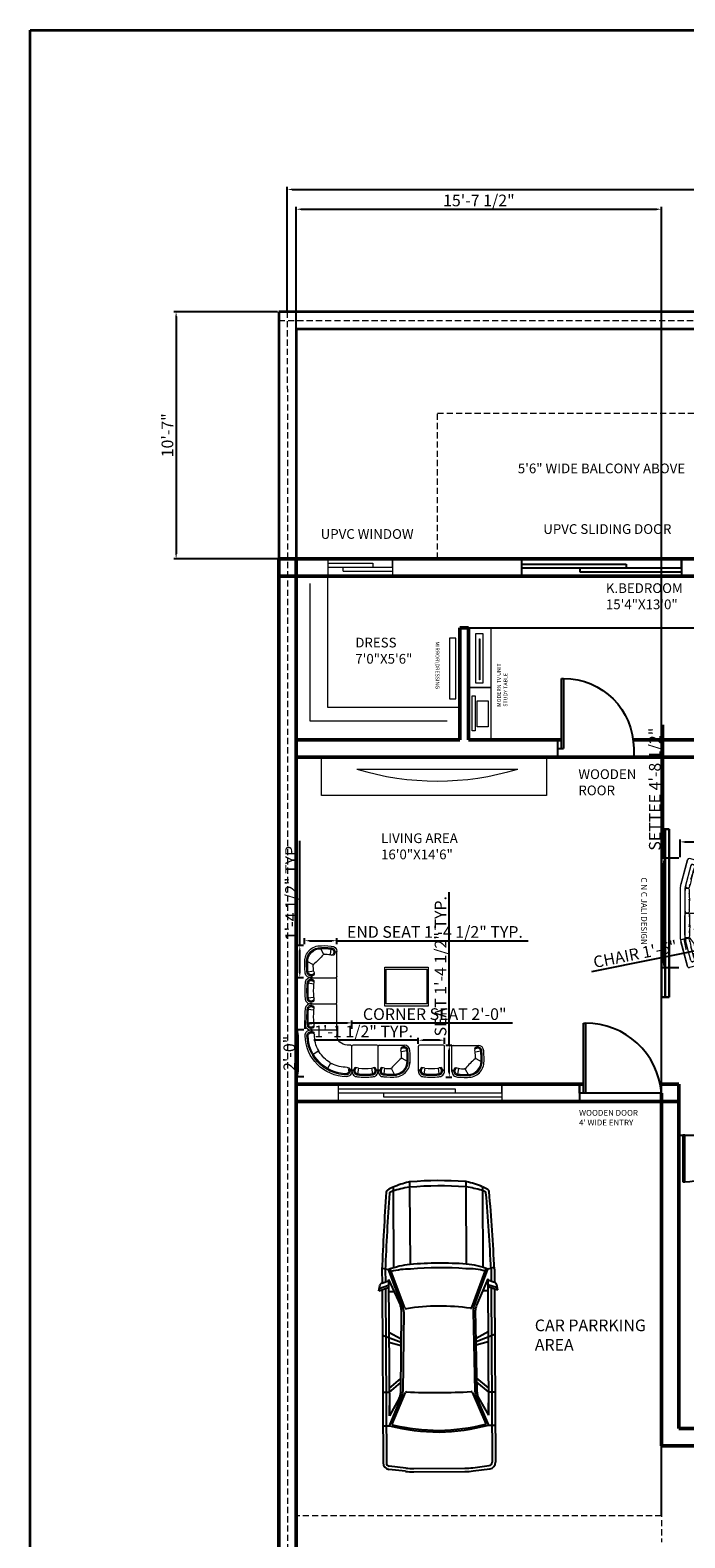
# Model space of a CAD drawing. Units: inches. Extents: x 2123 to 2977, y 1464 to 2698.
# Tile 2 of 10: x 2123 to 2459, y 1923 to 2698. Entities that reach past the tile are written whole.
import ezdxf

# ---------------------------------------------------------------- set-up
doc = ezdxf.new("R2010")
doc.units = ezdxf.units.IN
doc.linetypes.add('HIDDEN2', pattern=[4.7625, 3.175, -1.5875])
doc.layers.add('0 finos', color=250, linetype='Continuous')
for name, color, linetype, lineweight in [('A-ANNO-DIMS', 2, 'Continuous', 18), ('A-ANNO-TEXT', 7, 'Continuous', 18), ('A-ANNO-TTLB', 7, 'Continuous', 35), ('A-AREA-IDEN', 7, 'Continuous', 25), ('A-DOOR', 4, 'Continuous', 25), ('A-FLOR-OVHD', 253, 'HIDDEN2', 18), ('A-FURN', 8, 'Continuous', 18), ('A-FURN-FIXD', 8, 'Continuous', 20), ('A-GLAZ', 4, 'Continuous', 18), ('A-WALL', 7, 'Continuous', 50), ('A-WALL-PRTN', 7, 'Continuous', 30), ('C-PKNG-VEHC', 8, 'Continuous', 18), ('C-PROP', 21, 'HIDDEN2', 18), ('L-SITE-WALL', 7, 'Continuous', 35)]:
    doc.layers.add(name, color=color, linetype=linetype, lineweight=lineweight)
doc.styles.get("Standard").update_dxf_attribs({"font": 'arial.ttf'})
doc.dimstyles.new('ISO-25', dxfattribs={"dimtxt": 6, "dimasz": 2.5, "dimexe": 1.25, "dimexo": 0.625, "dimtad": 1, "dimdec": 0, "dimlunit": 3, "dimtxsty": 'Standard', "dimcen": 2.5, "dimadec": 0, "dimazin": 0, "dimtfac": 1, "dimtdec": 0, "dimtmove": 0, "dimatfit": 3, "dimfxl": 1, "dimarcsym": 0})

# ---------------------------------------------------------------- blocks, each defined once
blk = doc.blocks.new('carro')
at = {"layer": '0 finos'}
for p, q in [((-1.274, 0.841), (-1.249, 0.743)), ((-0.666, 0.502), (-1.258, 0.718)), ((-0.674, 0.532), (-1.249, 0.743)), ((-1.246, 0.843), (-1.047, 0.844)), ((-1.246, 0.793), (-1.063, 0.794)), ((-1.099, 0.744), (0.965, 0.756)), ((-1.099, 0.744), (-0.702, 0.571)), ((-1.045, 0.847), (-1.079, 0.744)), ((-0.964, 0.889), (-1.011, 0.744)), ((-0.93, 0.895), (-1.007, 0.881)), ((-0.93, 0.895), (-0.979, 0.744)), ((-0.963, 0.794), (1.676, 0.81)), ((-0.947, 0.845), (1.676, 0.86)), ((-0.919, 0.745), (-0.919, 0.665)), ((-0.299, 0.748), (-0.198, 0.565)), ((-0.258, 0.849), (-0.148, 0.566)), ((-0.149, 0.749), (-0.098, 0.567)), ((0.551, 0.753), (0.402, 0.577)), ((0.61, 0.754), (0.462, 0.578)), ((0.61, 0.754), (0.609, 0.854)), ((0.616, 0.508), (1.094, 0.714)), ((0.669, 0.564), (1.115, 0.756)), ((0.701, 0.605), (0.965, 0.756)), ((0.965, 0.756), (0.778, 0.755)), ((1.115, 0.756), (1.114, 0.856)), ((1.759, 0.516), (1.726, 0.766)), ((1.809, 0.522), (1.776, 0.773)), ((-2.494, 0.661), (-2.439, 0.661)), ((-2.439, 0.661), (-1.275, 0.668)), ((0.615, 0.581), (-0.626, 0.557)), ((-0.608, 0.521), (0.602, 0.549)), ((-2.573, 0.41), (-2.493, 0.411)), ((-2.476, 0.411), (-1.323, 0.417)), ((1.771, -0.377), (1.767, 0.398)), ((1.821, -0.377), (1.817, 0.398)), ((-2.568, -0.44), (-2.488, -0.439)), ((-2.471, -0.439), (-1.318, -0.433)), ((-2.432, -0.689), (-1.267, -0.682)), ((-0.661, -0.51), (-1.25, -0.733)), ((-0.668, -0.54), (-1.241, -0.757)), ((-1.091, -0.756), (-0.695, -0.579)), ((-0.911, -0.755), (-0.911, -0.676)), ((0.622, -0.574), (-0.62, -0.564)), ((-0.602, -0.528), (0.608, -0.542)), ((-0.291, -0.752), (-0.192, -0.567)), ((-0.248, -0.851), (-0.142, -0.568)), ((-0.141, -0.751), (-0.092, -0.568)), ((0.559, -0.747), (0.408, -0.572)), ((0.619, -0.746), (0.468, -0.573)), ((1.102, -0.701), (0.622, -0.501)), ((1.124, -0.743), (0.676, -0.556)), ((0.708, -0.597), (0.974, -0.744)), ((1.765, -0.495), (1.735, -0.746)), ((1.814, -0.501), (1.785, -0.752)), ((-2.487, -0.689), (-2.432, -0.689)), ((-1.262, -0.856), (-1.241, -0.757)), ((-1.237, -0.807), (-1.054, -0.806)), ((-1.236, -0.857), (-1.037, -0.856)), ((-1.091, -0.756), (0.974, -0.744)), ((-1.036, -0.859), (-1.071, -0.756)), ((-0.953, -0.9), (-1.002, -0.756)), ((-0.92, -0.905), (-0.996, -0.892)), ((-0.92, -0.905), (-0.971, -0.756)), ((-0.954, -0.806), (1.686, -0.79)), ((-0.937, -0.855), (1.686, -0.84)), ((0.619, -0.746), (0.619, -0.846)), ((0.974, -0.744), (0.819, -0.745)), ((1.124, -0.843), (1.124, -0.743))]:
    blk.add_line(p, q, dxfattribs=at)
for centre, radius, start, end in [((-2.14, 0.534), 0.376, 145.8602, 160.2963), ((-2.414, 0.72), 0.045, 99.6056, 145.8602), ((-2.25, 0.596), 0.2, 150.5092, 164.4728), ((-2.14, 0.534), 0.326, 147.5998, 150.5092), ((0.535, -34.533), 35.421, 92.8817, 94.7876), ((-2.403, 0.7), 0.015, 94.7595, 147.5998), ((0.535, -34.583), 35.421, 92.8817, 94.7595), ((-0.078, 0.306), 1.25, 159.5351, 174.8753), ((-0.049, 0.42), 1.205, 166.3495, 180.3763), ((-0.998, 0.832), 0.05, 100.189, 161.8979), ((1.096, 0.709), 0.005, 13.9297, 113.3542), ((-2.008, -0.06), 3.203, 1.1964, 13.9297), ((-2.008, -0.06), 3.228, 1.1964, 14.6587), ((1.677, 0.76), 0.1, 7.4579, 90.3329), ((1.677, 0.76), 0.05, 7.4579, 90.3329), ((-1.339, 0.159), 1.259, 156.5474, 167.8615), ((-0.601, 0.138), 1.911, 164.4728, 171.5741), ((-0.63, 0.737), 0.18, 246.5804, 271.1487), ((2.517, 0.015), 3.205, 171.6477, 189.0181), ((-0.612, 0.701), 0.18, 249.9002, 271.3224), ((-0.673, 0.483), 0.02, 351.6477, 69.9002), ((0.598, 0.729), 0.18, 271.3224, 293.3542), ((0.622, 0.494), 0.015, 113.3542, 183.6852), ((-5.6, 0.093), 6.22, 359.1748, 3.6852), ((0.612, 0.761), 0.18, 271.1487, 299.704), ((0.817, 0.392), 0.95, 0.3329, 7.4579), ((0.817, 0.392), 1, 0.3329, 7.4579), ((2.688, 0.016), 5.275, 175.8587, 184.807), ((-2.375, 0.382), 0.2, 167.8615, 175.8587), ((2.688, 0.016), 5.195, 175.7191, 184.9467), ((-2.294, 0.389), 0.2, 171.5741, 175.7191), ((3.848, 0.022), 5.186, 175.6321, 185.0337), ((3.848, 0.022), 5.116, 175.6321, 185.0337), ((-5.599, -0.158), 6.22, 356.9806, 1.4909), ((-2.008, 0.037), 3.203, 346.7361, 359.4694), ((-2.008, 0.037), 3.228, 346.0071, 359.4694), ((-2.37, -0.41), 0.2, 184.807, 192.8043), ((-1.337, -0.175), 1.259, 192.8043, 204.1184), ((-2.289, -0.415), 0.2, 184.9467, 189.0917), ((-0.6, -0.145), 1.911, 189.0917, 196.7185), ((-0.074, -0.307), 1.25, 185.7904, 201.1307), ((-0.044, -0.42), 1.205, 180.2895, 194.3163), ((0.822, -0.383), 0.95, 353.2079, 0.3329), ((0.822, -0.383), 1, 353.2079, 0.3329), ((-0.621, -0.744), 0.18, 89.5171, 114.0853), ((-0.604, -0.708), 0.18, 89.3433, 110.7656), ((-0.668, -0.491), 0.02, 290.7656, 9.0181), ((0.606, -0.722), 0.18, 67.3115, 89.3433), ((0.628, -0.487), 0.015, 176.9806, 247.3115), ((0.621, -0.754), 0.18, 60.9617, 89.5171), ((-2.134, -0.558), 0.376, 200.3694, 214.8056), ((-2.406, -0.748), 0.045, 214.8056, 261.0602), ((-2.406, -0.687), 0.025, 196.7185, 205.3192), ((-2.134, -0.558), 0.326, 205.3192, 213.066), ((0.133, 34.537), 35.421, 265.8782, 267.7841), ((-2.395, -0.728), 0.015, 213.066, 265.9063), ((0.133, 34.587), 35.421, 265.9063, 267.7841), ((-0.988, -0.843), 0.05, 198.7678, 260.4768), ((1.104, -0.697), 0.005, 247.3115, 346.7361), ((1.685, -0.74), 0.05, 270.3329, 353.2079), ((1.685, -0.74), 0.1, 270.3329, 353.2079)]:
    blk.add_arc(centre, radius, start, end, dxfattribs=at)
blk = doc.blocks.new('ДИВАН08')
for p, q in [((10, 838), (233, 1669)), ((233, 1669), (26, 897)), ((339, 1486), (160, 818)), ((777, 1575), (294, 1705)), ((1026, 1343), (400, 1521)), ((691, 1435), (619, 1433)), ((812, 1514), (787, 1417)), ((400, 1260), (453, 1348)), ((540, 1030), (740, 1020)), ((550, 1060), (830, 950)), ((910, 720), (1061, 1282)), ((0, 761), (0, -761)), ((150, 741), (150, -741)), ((480, 400), (800, 500)), ((900, 642), (900, -642)), ((310, 0), (900, 0)), ((780, 460), (580, 470)), ((600, -460), (430, -520)), ((10, -838), (233, -1669)), ((233, -1669), (26, -897)), ((339, -1486), (160, -818)), ((430, -500), (800, -530)), ((910, -720), (1061, -1282)), ((400, -1260), (453, -1348)), ((1026, -1343), (400, -1521)), ((500, -1100), (840, -1040)), ((800, -1020), (620, -1120)), ((777, -1575), (294, -1705)), ((691, -1435), (619, -1433)), ((812, -1514), (787, -1417))]:
    blk.add_line(p, q)
for centre, radius, start, end in [((281, 1656), 50, 75, 165), ((387, 1473), 50, 75, 165), ((362, 1495), 20, 89.0297, 94.7193), ((359, 1330), 185, 60.9703, 89.0297), ((439, 1474), 20, 345, 60.9703), ((764, 1527), 50, 345, 75), ((-610, 1509), 1045, 334.4223, 341.4421), ((298, 1228), 90.2, 326.9449, 350.757), ((1013, 1295), 50, 345, 75), ((300, 761), 300, 165, 180), ((450, 741), 300, 165, 180), ((242, 847), 72.2, 156.1517, 210.7358), ((269, 972), 185, 240.9703, 269.0297), ((266, 807), 20, 269.0297, 345), ((-57, 544), 353, 1.9165, 10.4824), ((213, 880), 92.8, 338.027, 9.0149), ((1200, 642), 300, 165, 180), ((86, 55), 209, 1.7155, 15.9571), ((-23, 353), 322, 358.4137, 13.7556), ((86, -55), 209, 344.0429, 358.2845), ((-23, -353), 322, 346.2444, 1.5863), ((300, -761), 300, 180, 195), ((450, -741), 300, 180, 195), ((242, -847), 72.2, 149.2642, 203.8483), ((269, -972), 185, 90.9703, 119.0297), ((266, -807), 20, 15, 90.9703), ((-57, -544), 353, 349.5176, 358.0835), ((213, -880), 92.8, 350.9851, 21.973), ((1200, -642), 300, 180, 195), ((-610, -1509), 1045, 18.5579, 25.5777), ((298, -1228), 90.2, 9.243, 33.0551), ((1013, -1295), 50, 285, 15), ((281, -1656), 50, 195, 285), ((387, -1473), 50, 195, 285), ((362, -1495), 20, 265.2807, 270.9703), ((359, -1330), 185, 270.9703, 299.0297), ((439, -1474), 20, 299.0297, 15), ((764, -1527), 50, 285, 15)]:
    blk.add_arc(centre, radius, start, end)
for points, knots in [([(459, 1469), (452, 1440), (431, 1359), (378, 1199), (347, 1000), (304, 860), (286, 801)], [0, 0, 0, 0, 90.187713, 250.973361, 505.38742, 689.989893, 689.989893, 689.989893, 689.989893]), ([(398, 1251), (413, 1308), (433, 1384), (489, 1480), (588, 1481), (651, 1453), (691, 1435)], [0, 0, 0, 0, 182.307841, 236.159489, 312.31722, 446.240501, 446.240501, 446.240501, 446.240501]), ([(525, 1401), (539, 1407), (583, 1425), (652, 1391), (683, 1425), (691, 1435)], [0, 0, 0, 0, 44.660676, 140.870988, 176.926501, 176.926501, 176.926501, 176.926501]), ([(400, 1260), (417, 1265), (477, 1281), (481, 1367), (520, 1397), (525, 1401)], [0, 0, 0, 0, 50, 176.134878, 196.761653, 196.761653, 196.761653, 196.761653]), ([(156, 55), (155, 68), (151, 132), (151, 244), (150, 392), (154, 520), (148, 633), (153, 704), (162, 778), (223, 769), (278, 775), (303, 714), (290, 642), (303, 516), (300, 345), (298, 186), (295, 82), (296, 27), (255, 6), (217, 1), (173, 12), (157, 41), (156, 55)], [0, 0, 0, 0, 37.52683, 194.502639, 336.34661, 480.520736, 579.37384, 668.990026, 713.725273, 764.098689, 821.099919, 865.09763, 933.523372, 1043.042771, 1240.322997, 1451.300934, 1509.736774, 1565.888367, 1594.82446, 1636.840587, 1680.06496, 1722.682399, 1722.682399, 1722.682399, 1722.682399]), ([(156, -55), (155, -68), (151, -132), (151, -244), (150, -392), (154, -520), (148, -633), (153, -704), (162, -778), (223, -769), (278, -775), (303, -714), (290, -642), (303, -516), (300, -345), (298, -186), (295, -82), (296, -27), (255, -6), (217, -1), (173, -12), (157, -41), (156, -55)], [0, 0, 0, 0, 37.52683, 194.502639, 336.34661, 480.520736, 579.37384, 668.990026, 713.725273, 764.098689, 821.099919, 865.09763, 933.523372, 1043.042771, 1240.322997, 1451.300934, 1509.736774, 1565.888367, 1594.82446, 1636.840587, 1680.06496, 1722.682399, 1722.682399, 1722.682399, 1722.682399]), ([(459, -1469), (452, -1440), (431, -1359), (378, -1199), (347, -1000), (304, -860), (286, -801)], [0, 0, 0, 0, 90.187713, 250.973361, 505.38742, 689.989893, 689.989893, 689.989893, 689.989893]), ([(398, -1251), (413, -1308), (433, -1384), (489, -1480), (588, -1481), (651, -1453), (691, -1435)], [0, 0, 0, 0, 182.307841, 236.159489, 312.31722, 446.240501, 446.240501, 446.240501, 446.240501]), ([(400, -1260), (417, -1265), (477, -1281), (481, -1367), (520, -1397), (525, -1401)], [0, 0, 0, 0, 50, 176.134878, 196.761653, 196.761653, 196.761653, 196.761653]), ([(525, -1401), (539, -1407), (583, -1425), (652, -1391), (683, -1425), (691, -1435)], [0, 0, 0, 0, 44.660676, 140.870988, 176.926501, 176.926501, 176.926501, 176.926501])]:
    blk.add_open_spline(points, degree=3, knots=knots)
blk = doc.blocks.new('A$C707258B2')
at = {"color": 0}
for p, q in [((0.404, 0.342), (1.074, 0.342)), ((0.404, 0.292), (0.454, 0.292)), ((0.404, 0.262), (0.454, 0.262)), ((1.104, 0.312), (1.104, 0.212)), ((0.6, -0.238), (0.47, -0.313)), ((1.479, -0.063), (1.379, -0.063)), ((1.509, -0.763), (1.509, -0.093)), ((0.929, -0.567), (0.854, -0.697)), ((1.429, -0.763), (1.429, -0.713)), ((1.459, -0.763), (1.459, -0.712))]:
    blk.add_line(p, q, dxfattribs=at)
for centre, radius, start, end in [((0.404, 0.192), 0.15, 90, 181.1754), ((1.379, 0.212), 1.125, 181.1754, 268.8246), ((0.404, 0.192), 0.1, 90, 181.1754), ((1.379, 0.212), 1.075, 181.1754, 208.6357), ((0.404, 0.192), 0.07, 90, 181.1754), ((1.379, 0.212), 1.045, 181.1754, 268.8246), ((0.378, 0.317), 0.0362, 316.3972, 43.6028), ((0.368, 0.317), 0.0662, 337.8298, 22.1702), ((0.455, 0.256), 0.0357, 345.4262, 90.5555), ((0.454, 0.212), 0.05, 360, 90), ((1.379, 0.212), 0.875, 180, 208.4082), ((1.074, 0.312), 0.03, 360, 90), ((1.379, 0.212), 0.275, 180, 270), ((0.457, -0.291), 0.025, 208.6357, 300), ((0.482, -0.334), 0.025, 120, 211.3643), ((1.379, 0.212), 1.075, 211.3643, 238.6357), ((0.587, -0.216), 0.025, 300, 28.4082), ((0.612, -0.259), 0.025, 31.5918, 120), ((1.379, 0.212), 0.875, 211.5918, 238.4082), ((1.479, -0.093), 0.03, 360, 90), ((0.832, -0.685), 0.025, 238.6357, 330), ((0.876, -0.71), 0.025, 150, 241.3643), ((1.379, 0.212), 1.075, 241.3643, 268.8246), ((0.907, -0.555), 0.025, 330, 58.4082), ((0.951, -0.58), 0.025, 61.5918, 150), ((1.379, 0.212), 0.875, 241.5918, 270), ((1.359, -0.763), 0.15, 268.8246, 360), ((1.359, -0.763), 0.1, 268.8246, 360), ((1.359, -0.763), 0.07, 268.8246, 360), ((1.379, -0.713), 0.05, 360, 90), ((1.425, -0.709), 0.0336, 354.6301, 109.3883), ((1.484, -0.799), 0.0662, 67.8298, 112.1702), ((1.484, -0.789), 0.0362, 46.3972, 133.6028)]:
    blk.add_arc(centre, radius, start, end, dxfattribs=at)
blk = doc.blocks.new('part 01')
at = {"color": 0}
for p, q in [((-591, 527), (-740, 550)), ((-670, 700), (0, 700)), ((-591, 527), (-579, 561)), ((30, 30), (30, 670)), ((-591, 173), (-740, 150)), ((-670, 0), (0, 0)), ((-591, 173), (-579, 139))]:
    blk.add_line(p, q, dxfattribs=at)
for centre, radius, start, end in [((1178, 350), 2008, 174.2835, 185.7165), ((-670, 550), 150, 90, 181.1754), ((1178, 350), 1958, 174.2835, 185.7165), ((-670, 550), 100, 90, 181.1754), ((1178, 350), 1928, 174.2835, 185.7165), ((-670, 550), 70, 90, 181.1754), ((-660, 518), 133, 56.0897, 95.6132), ((-696, 675), 36.2, 316.3972, 43.6028), ((-660, 518), 103, 42.0066, 95.6132), ((-706, 675), 66.2, 337.8298, 22.1702), ((1178, 350), 1778, 174.2835, 185.7165), ((-600, 607), 25, 332.9608, 56.0897), ((-625, 620), 53.2, 321.0017, 332.9608), ((-602, 570), 25, 340, 42.0066), ((0, 670), 30, 0, 90), ((-670, 150), 150, 178.8246, 270), ((-670, 150), 100, 178.8246, 270), ((-670, 150), 70, 178.8246, 270), ((-660, 182), 133, 264.3868, 303.9103), ((-660, 182), 103, 264.3868, 317.9934), ((-696, 25), 36.2, 316.3972, 43.6028), ((-706, 25), 66.2, 337.8298, 22.1702), ((-600, 93), 25, 303.9103, 27.0392), ((-602, 130), 25, 317.9934, 20), ((-625, 80), 53.2, 27.0392, 38.9983), ((0, 30), 30, 270, 0)]:
    blk.add_arc(centre, radius, start, end, dxfattribs=at)
blk = doc.blocks.new('part02')
at = {"color": 0}
for p, q in [((0, -670), (0, 0)), ((30, 30), (700, 30)), ((621, -143), (609, -109)), ((621, -143), (770, -120)), ((640, -326), (778, -399)), ((173, -591), (139, -579)), ((173, -591), (150, -740)), ((356, -610), (429, -748))]:
    blk.add_line(p, q, dxfattribs=at)
for centre, radius, start, end in [((30, 0), 30, 90, 180), ((726, 5), 56.2, 153.6122, 206.6666), ((726, 5), 36.2, 136.3972, 223.6028), ((700, -120), 150, 0, 90), ((2220, -2190), 2454, 130.6961, 139.3039), ((439, -409), 419, 268.2181, 1.7819), ((439, -409), 369, 268.2181, 1.7819), ((439, -409), 339, 268.2181, 1.7819), ((630, -63), 25, 123.9103, 207.0392), ((655, -50), 53.2, 207.0392, 218.9983), ((632, -100), 25, 137.9934, 200), ((690, -152), 103, 84.3868, 137.9934), ((689, -151), 132, 85.4378, 123.9887), ((632, -344), 20, 62, 130.6961), ((-1148, -320), 1778, 0.3836, 5.7165), ((650, -308), 20, 180.3836, 242), ((700, -121), 101, 357.5006, 89.858), ((700, -120), 70, 0, 90), ((-1228, -320), 2008, 357.7349, 5.7032), ((-1148, -320), 1958, 355.8657, 5.7165), ((-1148, -320), 2008, 355.818, 5.7165), ((25, -696), 56.2, 63.3334, 116.3878), ((25, -696), 36.2, 46.3972, 133.6028), ((150, -670), 150, 180, 271.1754), ((182, -660), 133, 146.0897, 185.6132), ((150, -670), 100, 180, 271.1754), ((93, -600), 25, 62.9608, 146.0897), ((182, -660), 103, 132.0066, 185.6132), ((150, -670), 70, 180, 270), ((80, -625), 53.2, 51.0017, 62.9608), ((130, -602), 25, 70, 132.0066), ((350, 1258), 2008, 264.2968, 272.2651), ((350, 1178), 1958, 264.2835, 274.1343), ((350, 1178), 1778, 264.2835, 269.6164), ((338, -620), 20, 28, 89.6164), ((374, -602), 20, 139.3039, 208), ((350, 1178), 2008, 264.2835, 274.182)]:
    blk.add_arc(centre, radius, start, end, dxfattribs=at)
blk = doc.blocks.new('*D11')
at = {"layer": 'A-ANNO-DIMS', "color": 0, "lineweight": -2, "transparency": 16777216}
for p, q in [((2255.34, 2553.5), (2255.34, 2617)), ((2257.84, 2615.75), (2759.66, 2615.75)), ((2762.16, 2553.5), (2762.16, 2617))]:
    blk.add_line(p, q, dxfattribs=at)
at = {"layer": 'A-ANNO-DIMS', "color": 0, "transparency": 16777216}
for points in [[(2257.84, 2616.16), (2257.84, 2615.33), (2255.34, 2615.75)], [(2759.66, 2616.16), (2759.66, 2615.33), (2762.16, 2615.75)]]:
    blk.add_solid(points, dxfattribs=at)
at = {"layer": 'Defpoints', "color": 0, "transparency": 16777216}
for p in [(2762.16, 2615.75), (2255.34, 2552.87), (2762.16, 2552.87)]:
    blk.add_point(p, dxfattribs=at)
at = {"layer": 'A-ANNO-DIMS', "color": 0, "transparency": 16777216, "insert": (2508.75, 2619.44), "char_height": 6, "attachment_point": 5}
blk.add_mtext('42\'-3"', dxfattribs=at)
blk = doc.blocks.new('SWING-DOOR-36')
for p, q in [((37, 36), (36, 36)), ((36, 36), (36, 0)), ((37, 0), (37, 36))]:
    blk.add_line(p, q)
blk.add_arc((36, 0), 36, 90, 180)
blk = doc.blocks.new('*D24')
at = {"layer": 'A-ANNO-DIMS', "color": 0, "lineweight": -2, "transparency": 16777216}
for p, q in [((2338.51, 2175.95), (2338.51, 2254.45)), ((2336.65, 2175.95), (2339.76, 2175.95)), ((2338.51, 2161.9), (2338.51, 2173.45)), ((2336.65, 2159.4), (2339.76, 2159.4))]:
    blk.add_line(p, q, dxfattribs=at)
at = {"layer": 'A-ANNO-DIMS', "color": 0, "transparency": 16777216}
for points in [[(2338.09, 2173.45), (2338.92, 2173.45), (2338.51, 2175.95)], [(2338.09, 2161.9), (2338.92, 2161.9), (2338.51, 2159.4)]]:
    blk.add_solid(points, dxfattribs=at)
at = {"layer": 'Defpoints', "color": 0, "transparency": 16777216}
for p in [(2336.03, 2175.95), (2338.51, 2175.95), (2336.03, 2159.4)]:
    blk.add_point(p, dxfattribs=at)
at = {"layer": 'A-ANNO-DIMS', "color": 0, "transparency": 16777216, "insert": (2334.78, 2216.45), "char_height": 6, "attachment_point": 5, "rotation": 90}
blk.add_mtext('SEAT 1\'-4 1/2" TYP.', dxfattribs=at)
blk = doc.blocks.new('*D25')
at = {"layer": 'A-ANNO-DIMS', "color": 0, "lineweight": -2, "transparency": 16777216}
for p, q in [((2322.61, 2178.43), (2268.87, 2178.43)), ((2322.61, 2176.57), (2322.61, 2179.68)), ((2333.53, 2178.43), (2325.11, 2178.43)), ((2336.03, 2176.57), (2336.03, 2179.68))]:
    blk.add_line(p, q, dxfattribs=at)
at = {"layer": 'A-ANNO-DIMS', "color": 0, "transparency": 16777216}
for points in [[(2325.11, 2178.85), (2325.11, 2178.01), (2322.61, 2178.43)], [(2333.53, 2178.85), (2333.53, 2178.01), (2336.03, 2178.43)]]:
    blk.add_solid(points, dxfattribs=at)
at = {"layer": 'Defpoints', "color": 0, "transparency": 16777216}
for p in [(2322.61, 2178.43), (2322.61, 2175.95), (2336.03, 2175.95)]:
    blk.add_point(p, dxfattribs=at)
at = {"layer": 'A-ANNO-DIMS', "color": 0, "transparency": 16777216, "insert": (2294.49, 2182.16), "char_height": 6, "attachment_point": 5}
blk.add_mtext('1\'-1 1/2" TYP.', dxfattribs=at)
blk = doc.blocks.new('*D26')
at = {"layer": 'A-ANNO-DIMS', "color": 0, "lineweight": -2, "transparency": 16777216}
for p, q in [((2264.21, 2227.71), (2264.21, 2230.82)), ((2266.71, 2229.57), (2278.26, 2229.57)), ((2280.76, 2227.71), (2280.76, 2230.82)), ((2280.76, 2229.57), (2378.99, 2229.57))]:
    blk.add_line(p, q, dxfattribs=at)
at = {"layer": 'A-ANNO-DIMS', "color": 0, "transparency": 16777216}
for points in [[(2266.71, 2229.99), (2266.71, 2229.15), (2264.21, 2229.57)], [(2278.26, 2229.99), (2278.26, 2229.15), (2280.76, 2229.57)]]:
    blk.add_solid(points, dxfattribs=at)
at = {"layer": 'Defpoints', "color": 0, "transparency": 16777216}
for p in [(2264.21, 2227.09), (2280.76, 2229.57), (2280.76, 2227.09)]:
    blk.add_point(p, dxfattribs=at)
at = {"layer": 'A-ANNO-DIMS', "color": 0, "transparency": 16777216, "insert": (2331.12, 2233.3), "char_height": 6, "attachment_point": 5}
blk.add_mtext('END SEAT 1\'-4 1/2" TYP.', dxfattribs=at)
blk = doc.blocks.new('*D27')
at = {"layer": 'A-ANNO-DIMS', "color": 0, "lineweight": -2, "transparency": 16777216}
for p, q in [((2261.73, 2227.09), (2261.73, 2280.83)), ((2263.59, 2227.09), (2260.48, 2227.09)), ((2261.73, 2213.05), (2261.73, 2224.59)), ((2263.59, 2210.55), (2260.48, 2210.55))]:
    blk.add_line(p, q, dxfattribs=at)
at = {"layer": 'A-ANNO-DIMS', "color": 0, "transparency": 16777216}
for points in [[(2261.32, 2224.59), (2262.15, 2224.59), (2261.73, 2227.09)], [(2261.32, 2213.05), (2262.15, 2213.05), (2261.73, 2210.55)]]:
    blk.add_solid(points, dxfattribs=at)
at = {"layer": 'Defpoints', "color": 0, "transparency": 16777216}
for p in [(2261.73, 2227.09), (2264.21, 2227.09), (2264.21, 2210.55)]:
    blk.add_point(p, dxfattribs=at)
at = {"layer": 'A-ANNO-DIMS', "color": 0, "transparency": 16777216, "insert": (2258.01, 2255.21), "char_height": 6, "attachment_point": 5, "rotation": 90}
blk.add_mtext('1\'-4 1/2" TYP.', dxfattribs=at)
blk = doc.blocks.new('*D28')
at = {"layer": 'A-ANNO-DIMS', "color": 0, "lineweight": -2, "transparency": 16777216}
for p, q in [((2264.45, 2184.34), (2264.45, 2188.57)), ((2266.95, 2187.32), (2286.02, 2187.32)), ((2288.52, 2184.34), (2288.52, 2188.57)), ((2288.52, 2187.32), (2371.02, 2187.32))]:
    blk.add_line(p, q, dxfattribs=at)
at = {"layer": 'A-ANNO-DIMS', "color": 0, "transparency": 16777216}
for points in [[(2266.95, 2187.74), (2266.95, 2186.91), (2264.45, 2187.32)], [(2286.02, 2187.74), (2286.02, 2186.91), (2288.52, 2187.32)]]:
    blk.add_solid(points, dxfattribs=at)
at = {"layer": 'Defpoints', "color": 0, "transparency": 16777216}
for p in [(2288.52, 2187.32), (2264.45, 2183.71), (2288.52, 2183.71)]:
    blk.add_point(p, dxfattribs=at)
at = {"layer": 'A-ANNO-DIMS', "color": 0, "transparency": 16777216, "insert": (2331.02, 2191.05), "char_height": 6, "attachment_point": 5}
blk.add_mtext('CORNER SEAT 2\'-0"', dxfattribs=at)
blk = doc.blocks.new('*D29')
at = {"layer": 'A-ANNO-DIMS', "color": 0, "lineweight": -2, "transparency": 16777216}
for p, q in [((2263.83, 2183.71), (2259.59, 2183.71)), ((2260.84, 2162.14), (2260.84, 2181.21)), ((2263.83, 2159.64), (2259.59, 2159.64))]:
    blk.add_line(p, q, dxfattribs=at)
at = {"layer": 'A-ANNO-DIMS', "color": 0, "transparency": 16777216}
for points in [[(2260.42, 2181.21), (2261.26, 2181.21), (2260.84, 2183.71)], [(2260.42, 2162.14), (2261.26, 2162.14), (2260.84, 2159.64)]]:
    blk.add_solid(points, dxfattribs=at)
at = {"layer": 'Defpoints', "color": 0, "transparency": 16777216}
for p in [(2260.84, 2183.71), (2264.45, 2183.71), (2264.45, 2159.64)]:
    blk.add_point(p, dxfattribs=at)
at = {"layer": 'A-ANNO-DIMS', "color": 0, "transparency": 16777216, "insert": (2257.15, 2171.68), "char_height": 6, "attachment_point": 5, "rotation": 90}
blk.add_mtext('2\'-0"', dxfattribs=at)
blk = doc.blocks.new('*D30')
at = {"layer": 'A-ANNO-DIMS', "color": 0, "lineweight": -2, "transparency": 16777216}
for p, q in [((2448.55, 2271.92), (2448.55, 2340.5)), ((2456.37, 2271.92), (2447.3, 2271.92)), ((2448.55, 2218.14), (2448.55, 2269.42)), ((2456.37, 2215.64), (2447.3, 2215.64))]:
    blk.add_line(p, q, dxfattribs=at)
at = {"layer": 'A-ANNO-DIMS', "color": 0, "transparency": 16777216}
for points in [[(2448.13, 2269.42), (2448.97, 2269.42), (2448.55, 2271.92)], [(2448.13, 2218.14), (2448.97, 2218.14), (2448.55, 2215.64)]]:
    blk.add_solid(points, dxfattribs=at)
at = {"layer": 'Defpoints', "color": 0, "transparency": 16777216}
for p in [(2448.55, 2271.92), (2456.99, 2271.92), (2456.99, 2215.64)]:
    blk.add_point(p, dxfattribs=at)
at = {"layer": 'A-ANNO-DIMS', "color": 0, "transparency": 16777216, "insert": (2444.82, 2307.46), "char_height": 6, "attachment_point": 5, "rotation": 90}
blk.add_mtext('SETTEE 4\'-8 1/2"', dxfattribs=at)
blk = doc.blocks.new('*D31')
at = {"layer": 'A-ANNO-DIMS', "color": 0, "lineweight": -2, "transparency": 16777216}
for p, q in [((2456.99, 2272.54), (2456.99, 2281.61)), ((2459.49, 2280.36), (2472.04, 2280.36)), ((2474.54, 2272.54), (2474.54, 2281.61)), ((2474.54, 2280.36), (2507.66, 2280.36))]:
    blk.add_line(p, q, dxfattribs=at)
at = {"layer": 'A-ANNO-DIMS', "color": 0, "transparency": 16777216}
for points in [[(2459.49, 2280.77), (2459.49, 2279.94), (2456.99, 2280.36)], [(2472.04, 2280.77), (2472.04, 2279.94), (2474.54, 2280.36)]]:
    blk.add_solid(points, dxfattribs=at)
at = {"layer": 'Defpoints', "color": 0, "transparency": 16777216}
for p in [(2474.54, 2280.36), (2456.99, 2271.92), (2474.54, 2271.92)]:
    blk.add_point(p, dxfattribs=at)
at = {"layer": 'A-ANNO-DIMS', "color": 0, "transparency": 16777216, "insert": (2492.35, 2284.08), "char_height": 6, "attachment_point": 5}
blk.add_mtext('1\'-5 1/2"', dxfattribs=at)
blk = doc.blocks.new('*D32')
at = {"layer": 'A-ANNO-DIMS', "color": 0, "lineweight": -2, "transparency": 16777216}
for p, q in [((2478.82, 2227.08), (2411.5, 2213.61)), ((2479.23, 2225.03), (2478.58, 2228.3)), ((2494.1, 2230.13), (2481.27, 2227.57)), ((2496.96, 2228.58), (2496.31, 2231.85))]:
    blk.add_line(p, q, dxfattribs=at)
at = {"layer": 'A-ANNO-DIMS', "color": 0, "transparency": 16777216}
for points in [[(2481.19, 2227.98), (2481.36, 2227.16), (2478.82, 2227.08)], [(2494.02, 2230.54), (2494.18, 2229.73), (2496.55, 2230.62)]]:
    blk.add_solid(points, dxfattribs=at)
at = {"layer": 'Defpoints', "color": 0, "transparency": 16777216}
for p in [(2478.82, 2227.08), (2479.36, 2224.42), (2497.08, 2227.96)]:
    blk.add_point(p, dxfattribs=at)
at = {"layer": 'A-ANNO-DIMS', "color": 0, "transparency": 16777216, "insert": (2443.2, 2223.76), "char_height": 6, "attachment_point": 5, "rotation": 11.30993}
blk.add_mtext('CHAIR 1\'-6" TYP.', dxfattribs=at)
blk = doc.blocks.new('*D54')
at = {"layer": 'A-ANNO-DIMS', "color": 0, "lineweight": -2, "transparency": 16777216}
for p, q in [((2250.31, 2552.87), (2196.99, 2552.87)), ((2198.24, 2550.37), (2198.24, 2428.37)), ((2250.31, 2425.87), (2196.99, 2425.87))]:
    blk.add_line(p, q, dxfattribs=at)
at = {"layer": 'A-ANNO-DIMS', "color": 0, "transparency": 16777216}
for points in [[(2197.82, 2550.37), (2198.65, 2550.37), (2198.24, 2552.87)], [(2197.82, 2428.37), (2198.65, 2428.37), (2198.24, 2425.87)]]:
    blk.add_solid(points, dxfattribs=at)
at = {"layer": 'Defpoints', "color": 0, "transparency": 16777216}
for p in [(2250.94, 2552.87), (2198.24, 2425.87), (2250.94, 2425.87)]:
    blk.add_point(p, dxfattribs=at)
at = {"layer": 'A-ANNO-DIMS', "color": 0, "transparency": 16777216, "insert": (2194.55, 2489.37), "char_height": 6, "attachment_point": 5, "rotation": 90}
blk.add_mtext('10\'-7"', dxfattribs=at)
blk = doc.blocks.new('*D56')
at = {"layer": 'A-ANNO-DIMS', "color": 0, "lineweight": -2, "transparency": 16777216}
for p, q in [((2259.94, 1934.5), (2259.94, 2606.82)), ((2262.44, 2605.57), (2444.94, 2605.57)), ((2447.44, 1934.5), (2447.44, 2606.82))]:
    blk.add_line(p, q, dxfattribs=at)
at = {"layer": 'A-ANNO-DIMS', "color": 0, "transparency": 16777216}
for points in [[(2262.44, 2605.99), (2262.44, 2605.15), (2259.94, 2605.57)], [(2444.94, 2605.99), (2444.94, 2605.15), (2447.44, 2605.57)]]:
    blk.add_solid(points, dxfattribs=at)
at = {"layer": 'Defpoints', "color": 0, "transparency": 16777216}
for p in [(2447.44, 2605.57), (2259.94, 1933.87), (2447.44, 1933.88)]:
    blk.add_point(p, dxfattribs=at)
at = {"layer": 'A-ANNO-DIMS', "color": 0, "transparency": 16777216, "insert": (2353.69, 2609.3), "char_height": 6, "attachment_point": 5}
blk.add_mtext('15\'-7 1/2"', dxfattribs=at)
blk = doc.blocks.new('*D59')
at = {"layer": 'A-ANNO-DIMS', "color": 0, "lineweight": -2, "transparency": 16777216}
for p, q in [((2819.64, 2416.87), (2819.64, 2450.65)), ((2376.14, 2416.87), (2820.89, 2416.87)), ((2819.64, 2392.84), (2819.64, 2414.37)), ((2344.56, 2390.34), (2820.89, 2390.34))]:
    blk.add_line(p, q, dxfattribs=at)
at = {"layer": 'A-ANNO-DIMS', "color": 0, "transparency": 16777216}
for points in [[(2819.22, 2414.37), (2820.05, 2414.37), (2819.64, 2416.87)], [(2819.22, 2392.84), (2820.05, 2392.84), (2819.64, 2390.34)]]:
    blk.add_solid(points, dxfattribs=at)
at = {"layer": 'Defpoints', "color": 0, "transparency": 16777216}
for p in [(2375.52, 2416.87), (2819.64, 2416.87), (2343.94, 2390.34)]:
    blk.add_point(p, dxfattribs=at)
at = {"layer": 'A-ANNO-DIMS', "color": 0, "transparency": 16777216, "insert": (2815.91, 2435.01), "char_height": 6, "attachment_point": 5, "rotation": 90}
blk.add_mtext('2\'-2 1/2"', dxfattribs=at)

msp = doc.modelspace()

# ---------------------------------------------------------------- linework, layer by layer
at = {"layer": 'A-ANNO-TTLB'}
msp.add_lwpolyline([(2123.3, 2697.62), (2977.18, 2697.62), (2977.18, 1463.53), (2123.3, 1463.53)], close=True, dxfattribs=at)
at = {"layer": 'A-DOOR'}
for p, q in [((2375.52, 2425.87), (2375.52, 2416.87)), ((2457.7, 2421.16), (2457.7, 2425.87)), ((2457.7, 2425.87), (2457.7, 2416.87)), ((2375.52, 2423.16), (2429.32, 2423.16)), ((2375.52, 2423.16), (2429.32, 2423.16)), ((2375.52, 2421.16), (2457.7, 2421.16)), ((2405.5, 2421.16), (2405.5, 2419.16)), ((2405.5, 2419.16), (2457.7, 2419.16)), ((2429.32, 2423.16), (2429.32, 2421.16)), ((2394.19, 2323.87), (2394.19, 2332.87)), ((2394.19, 2328.37), (2397.19, 2328.37)), ((2433.19, 2328.37), (2433.19, 2323.87)), ((2407.44, 2151.25), (2407.44, 2187.25)), ((2407.44, 2187.25), (2408.44, 2187.25)), ((2408.44, 2187.25), (2408.44, 2151.25)), ((2405.44, 2151.25), (2405.44, 2155.87)), ((2405.44, 2155.87), (2405.44, 2146.87)), ((2407.44, 2151.25), (2405.44, 2151.25)), ((2409.44, 2151.25), (2407.44, 2151.25)), ((2407.44, 2151.25), (2407.44, 2151.25)), ((2445.44, 2151.25), (2409.44, 2151.25)), ((2447.44, 2151.25), (2445.44, 2151.25)), ((2456.44, 2129.62), (2458.44, 2129.62)), ((2458.44, 2129.62), (2458.44, 2105.59)), ((2459.44, 2129.62), (2458.44, 2129.62)), ((2458.44, 2129.62), (2458.44, 2129.62)), ((2458.44, 2129.62), (2485.24, 2129.62)), ((2459.44, 2105.59), (2459.44, 2129.62)), ((2459.44, 2129.62), (2459.44, 2129.62)), ((2458.44, 2105.59), (2459.44, 2105.59))]:
    msp.add_line(p, q, dxfattribs=at)
for centre, radius, start, end in [((2408.44, 2148.13), 39.12, 4.58122, 90), ((2459.44, 2131.47), 25.87, 270, 355.91159)]:
    msp.add_arc(centre, radius, start, end, dxfattribs=at)
at = {"layer": 'A-FLOR-OVHD'}
for p, q in [((2332.44, 2425.87), (2332.44, 2500.76)), ((2332.44, 2500.76), (2535.66, 2500.76)), ((2447.44, 1969.87), (2447.44, 1920.38)), ((2447.44, 1933.88), (2259.94, 1933.87))]:
    msp.add_line(p, q, dxfattribs=at)
at = {"layer": 'A-FURN'}
for points in [[(2305.38, 2215.91), (2327.69, 2215.91), (2327.69, 2195.95), (2305.38, 2195.95)], [(2306.03, 2215.01), (2327.01, 2215.01), (2327.01, 2197.08), (2306.03, 2197.08)]]:
    msp.add_lwpolyline(points, close=True, dxfattribs=at)
at = {"layer": 'A-FURN-FIXD'}
for p, q in [((2266.94, 2413.22), (2266.94, 2342.57)), ((2354.05, 2363.74), (2354.05, 2384.75)), ((2354.05, 2384.75), (2354.27, 2384.75)), ((2354.27, 2384.75), (2354.27, 2363.74)), ((2354.27, 2363.74), (2354.05, 2363.74)), ((2266.94, 2342.57), (2337.41, 2342.57)), ((2291.02, 2317.8), (2373.65, 2317.8))]:
    msp.add_line(p, q, dxfattribs=at)
for points in [[(2259.94, 2349.62), (2259.94, 2416.87), (2275.95, 2416.87), (2275.95, 2349.62)], [(2275.95, 2349.62), (2343.94, 2349.62), (2343.94, 2332.87), (2275.95, 2332.87)]]:
    msp.add_lwpolyline(points, dxfattribs=at)
for points in [[(2348.44, 2390.34), (2359.83, 2390.34), (2359.83, 2332.87), (2348.44, 2332.87)], [(2352.22, 2387.5), (2355.76, 2387.5), (2355.76, 2361.96), (2352.22, 2361.96)], [(2341.83, 2385.08), (2338.69, 2385.08), (2338.69, 2353.92), (2341.83, 2353.92)], [(2348.44, 2359.66), (2359.83, 2359.66), (2359.83, 2359.66), (2348.44, 2359.66)], [(2350.17, 2355.41), (2351.71, 2355.41), (2351.71, 2337.46), (2350.17, 2337.46)], [(2352.83, 2352.88), (2358.46, 2352.88), (2358.46, 2339.49), (2352.83, 2339.49)], [(2272.95, 2323.87), (2388.39, 2323.87), (2388.39, 2304.28), (2272.95, 2304.28)]]:
    msp.add_lwpolyline(points, close=True, dxfattribs=at)
msp.add_arc((2332.33, 2452.83), 141.2, 252.98658, 287.01342, dxfattribs=at)
at = {"layer": 'A-GLAZ'}
for p, q in [((2276.07, 2425.87), (2276.07, 2416.87)), ((2309.39, 2421.57), (2309.39, 2425.87)), ((2309.39, 2425.87), (2309.39, 2416.87)), ((2276.07, 2423.57), (2299.33, 2423.57)), ((2276.07, 2421.57), (2309.39, 2421.57)), ((2283.98, 2419.57), (2283.98, 2421.57)), ((2283.98, 2419.57), (2309.39, 2419.57)), ((2299.33, 2423.57), (2299.33, 2421.57)), ((2309.39, 2423.57), (2309.39, 2421.57)), ((2309.39, 2421.57), (2309.39, 2423.57)), ((2309.39, 2423.57), (2309.39, 2423.57)), ((2309.39, 2423.57), (2309.39, 2423.57)), ((2281.53, 2155.87), (2281.53, 2146.87)), ((2365.53, 2151.37), (2365.53, 2155.87)), ((2365.53, 2155.87), (2365.53, 2146.87)), ((2281.53, 2153.37), (2341.53, 2153.37)), ((2281.53, 2151.37), (2341.53, 2151.37)), ((2304.69, 2151.37), (2304.69, 2149.37)), ((2304.69, 2149.37), (2341.53, 2149.37)), ((2341.53, 2153.37), (2341.53, 2151.37)), ((2341.53, 2151.37), (2365.53, 2151.37)), ((2341.53, 2149.37), (2365.53, 2149.37))]:
    msp.add_line(p, q, dxfattribs=at)
at = {"layer": 'A-WALL'}
for p, q in [((2250.94, 2425.87), (2250.94, 1969.87)), ((2250.94, 2425.87), (2766.94, 2425.87)), ((2259.94, 2425.87), (2259.94, 2332.87)), ((2250.94, 2416.87), (2687.94, 2416.87)), ((2343.94, 2390.34), (2348.44, 2390.34)), ((2343.94, 2390.34), (2343.94, 2332.87)), ((2348.44, 2390.34), (2348.44, 2332.87)), ((2259.94, 2332.87), (2343.94, 2332.87)), ((2259.94, 2332.87), (2343.94, 2332.87)), ((2259.94, 2332.87), (2259.94, 2323.87)), ((2348.44, 2332.87), (2396.19, 2332.87)), ((2348.44, 2332.87), (2396.19, 2332.87)), ((2432.9, 2332.87), (2537.44, 2332.87)), ((2259.94, 2323.87), (2537.44, 2323.87)), ((2259.94, 2323.87), (2259.94, 1969.87)), ((2259.94, 2155.87), (2407.44, 2155.87)), ((2446.79, 2155.87), (2456.44, 2155.87)), ((2456.44, 2155.87), (2456.44, 1978.87)), ((2259.94, 2146.87), (2456.44, 2146.87)), ((2447.44, 2151.25), (2447.44, 1969.87)), ((2456.44, 1978.87), (2685.94, 1978.87)), ((2250.94, 1969.87), (2250.94, 1909.87)), ((2259.94, 1897.87), (2259.94, 1969.87)), ((2447.44, 1969.87), (2685.94, 1969.87))]:
    msp.add_line(p, q, dxfattribs=at)
at = {"layer": 'A-WALL-PRTN'}
for p, q in [((2447.44, 2200.49), (2447.44, 2286.93)), ((2447.44, 2286.93), (2449.44, 2286.93)), ((2449.44, 2286.93), (2451.44, 2286.93)), ((2449.44, 2286.93), (2449.44, 2200.48)), ((2451.44, 2286.93), (2451.44, 2200.47)), ((2451.44, 2200.47), (2447.44, 2200.49))]:
    msp.add_line(p, q, dxfattribs=at)
at = {"layer": 'C-PROP'}
for p, q in [((2255.34, 2552.87), (2255.44, 1683.96)), ((2250.94, 2548.37), (2250.94, 2548.37)), ((2250.94, 2548.37), (2766.94, 2548.37))]:
    msp.add_line(p, q, dxfattribs=at)
at = {"layer": 'L-SITE-WALL'}
for p, q in [((2766.94, 2552.87), (2250.94, 2552.87)), ((2250.94, 2552.87), (2250.94, 2425.87)), ((2250.94, 2552.87), (2250.94, 2548.37)), ((2757.94, 2543.87), (2259.94, 2543.87)), ((2259.94, 2543.87), (2259.94, 2425.87))]:
    msp.add_line(p, q, dxfattribs=at)

# ---------------------------------------------------------------- block references
at = {"layer": 'A-DOOR', "extrusion": (0, 0, -1), "zscale": -1}
msp.add_blockref('SWING-DOOR-36', (-2433.19, 2328.37), dxfattribs=at)
at = {"layer": 'A-FURN', "xscale": 0.0164364890095425, "yscale": 0.0164364890095425, "zscale": 0.0164364890095425}
msp.add_blockref('ДИВАН08', (2456.99, 2243.78), dxfattribs=at)
at = {"layer": 'A-FURN', "ltscale": 0.03}
for name, p, xscale, yscale, zscale, rotation in [('part02', (2280.18, 2210.55), -0.0191689539784662, 0.0191689539784662, 0.0191689539784662, 269.9999999999968), ('A$C707258B2', (2281.96, 2154.79), -19.1689539784662, 19.1689539784662, 19.1689539784662, 269.9999999999968), ('part 01', (2301.94, 2175.37), 0.0191689539784662, 0.0191689539784662, 0.0191689539784662, 90), ('part 01', (2336.03, 2175.37), 0.0191689539784662, 0.0191689539784662, 0.0191689539784662, 90)]:
    msp.add_blockref(name, p, dxfattribs=dict(at, xscale=xscale, yscale=yscale, zscale=zscale, rotation=rotation))
at = {"layer": 'A-FURN', "ltscale": 0.03, "xscale": 0.0191689539784662, "yscale": 0.0191689539784662, "zscale": 0.0191689539784662}
for name, p in [('part 01', (2280.18, 2197.13)), ('part 01', (2280.18, 2183.71)), ('part02', (2301.94, 2175.37)), ('part02', (2339.89, 2175.21))]:
    msp.add_blockref(name, p, dxfattribs=at)
at = {"layer": 'C-PKNG-VEHC', "xscale": 33.95074894597202, "yscale": 33.95074894597202, "zscale": 33.95074894597202, "rotation": 270}
msp.add_blockref('carro', (2333.04, 2018.41), dxfattribs=at)

# ---------------------------------------------------------------- texts
at = {"layer": 'A-ANNO-TEXT', "attachment_point": 1}
for s, width, insert, char_height in [('5\'6" WIDE BALCONY ABOVE', 145.352, (2373.69, 2474.85), 5), ('UPVC WINDOW', 116.1895, (2272.46, 2441.14), 5), ('UPVC SLIDING DOOR', 154.7653, (2386.76, 2443.67), 5), ('WOODEN \\PROOR', 69.1443, (2404.8, 2317.67), 5), ("WOODEN DOOR\\P4' WIDE ENTRY", 79.7644, (2405.14, 2142.59), 3)]:
    msp.add_mtext_dynamic_manual_height_columns(s, width=width, gutter_width=12.5, heights=[0], dxfattribs=dict(at, insert=insert, char_height=char_height))
for s, width, insert, char_height, rotation in [('MIRROR\\\\DRESSING', 90.1653, (2333.44, 2383.4), 2, 270), ('MODERN TV UNIT\\PSTUDY TABLE', 123.6084, (2363.01, 2349.85), 2, 90), ('C N C JALI DESIGN', 134.7364, (2440.02, 2262.08), 3, 270)]:
    msp.add_mtext_dynamic_manual_height_columns(s, width=width, gutter_width=12.5, heights=[0], dxfattribs=dict(at, insert=insert, char_height=char_height, rotation=rotation))
at = {"layer": 'A-AREA-IDEN', "attachment_point": 1}
for s, width, insert, char_height in [('K.BEDROOM\\P15\'4"X13\'0"', 140.2678, (2418.92, 2413.3), 5), ('DRESS\\P7\'0"X5\'6"', 150.4746, (2290.24, 2385.31), 5), ('LIVING AREA\\P16\'0"X14\'6"', 393.6049, (2303.45, 2284.75), 5), ('CAR PARRKING\\PAREA', 307.4027, (2382.42, 2034.85), 6)]:
    msp.add_mtext_dynamic_manual_height_columns(s, width=width, gutter_width=12.5, heights=[0], dxfattribs=dict(at, insert=insert, char_height=char_height))

# ---------------------------------------------------------------- dimensions: what is measured, and where the dimension line sits
at = {"layer": 'A-ANNO-DIMS'}
for base, p1, p2, override, picture, middle in [((2762.16, 2615.75), (2255.34, 2552.87), (2762.16, 2552.87), {"dimclrd": 0, "dimclre": 0, "dimclrt": 0}, '*D11', (2508.75, 2619.44)), ((2447.44, 2605.57), (2259.94, 1933.87), (2447.44, 1933.88), {"dimdec": 1, "dimlfac": 1, "dimrnd": 0, "dimzin": 1, "dimdsep": 46, "dimlunit": 4, "dimfrac": 2}, '*D56', (2353.69, 2609.3)), ((2474.5449, 2280.3563), (2456.9906, 2271.9153), (2474.5449, 2271.9153), {"dimdec": 1, "dimlfac": 1, "dimrnd": 0, "dimzin": 1, "dimdsep": 46, "dimlunit": 4, "dimfrac": 2}, '*D31', (2492.3527, 2284.0836))]:
    dim = msp.add_linear_dim(base=base, p1=p1, p2=p2, dimstyle='ISO-25', override=override, dxfattribs=at)
    dim.commit()
    dim.dimension.update_dxf_attribs({"geometry": picture, "text_midpoint": middle})
for base, p1, p2, picture, middle in [((2198.24, 2425.87), (2250.94, 2552.87), (2250.94, 2425.87), '*D54', (2194.55, 2489.37)), ((2819.64, 2416.87), (2343.94, 2390.34), (2375.52, 2416.87), '*D59', (2815.91, 2435.01)), ((2260.84, 2183.71), (2264.45, 2159.64), (2264.45, 2183.71), '*D29', (2257.15, 2171.68))]:
    dim = msp.add_linear_dim(base=base, p1=p1, p2=p2, angle=90, dimstyle='ISO-25', override={"dimdec": 1, "dimlfac": 1, "dimrnd": 0, "dimzin": 1, "dimdsep": 46, "dimlunit": 4, "dimfrac": 2}, dxfattribs=at)
    dim.commit()
    dim.dimension.update_dxf_attribs({"geometry": picture, "text_midpoint": middle})
for base, p1, p2, angle, text, picture, middle in [((2448.55, 2271.92), (2456.99, 2215.64), (2456.99, 2271.92), 90, 'SETTEE <>', '*D30', (2444.82, 2307.46)), ((2261.73, 2227.09), (2264.21, 2210.55), (2264.21, 2227.09), 90, '<> TYP.', '*D27', (2258.01, 2255.21)), ((2338.5073, 2175.9492), (2336.0256, 2159.4043), (2336.0256, 2175.9492), 90, 'SEAT <> TYP.', '*D24', (2334.78, 2216.4473)), ((2478.82, 2227.08), (2497.08, 2227.96), (2479.36, 2224.42), 191.30993, 'CHAIR <> TYP.', '*D32', (2443.2, 2223.76)), ((2322.61, 2178.43), (2336.03, 2175.95), (2322.61, 2175.95), 180, '<> TYP.', '*D25', (2294.49, 2182.16))]:
    dim = msp.add_linear_dim(base=base, p1=p1, p2=p2, angle=angle, text=text, dimstyle='ISO-25', override={"dimdec": 1, "dimlfac": 1, "dimrnd": 0, "dimzin": 1, "dimdsep": 46, "dimlunit": 4, "dimfrac": 2}, dxfattribs=at)
    dim.commit()
    dim.dimension.update_dxf_attribs({"geometry": picture, "text_midpoint": middle})
for base, p1, p2, text, picture, middle in [((2280.755, 2229.5706), (2264.2147, 2227.0895), (2280.755, 2227.0895), 'END SEAT <> TYP.', '*D26', (2331.1228, 2233.2979)), ((2288.52, 2187.32), (2264.45, 2183.71), (2288.52, 2183.71), 'CORNER SEAT <>', '*D28', (2331.02, 2191.05))]:
    dim = msp.add_linear_dim(base=base, p1=p1, p2=p2, text=text, dimstyle='ISO-25', override={"dimdec": 1, "dimlfac": 1, "dimrnd": 0, "dimzin": 1, "dimdsep": 46, "dimlunit": 4, "dimfrac": 2}, dxfattribs=at)
    dim.commit()
    dim.dimension.update_dxf_attribs({"geometry": picture, "text_midpoint": middle})

doc.saveas('drawing.dxf')
